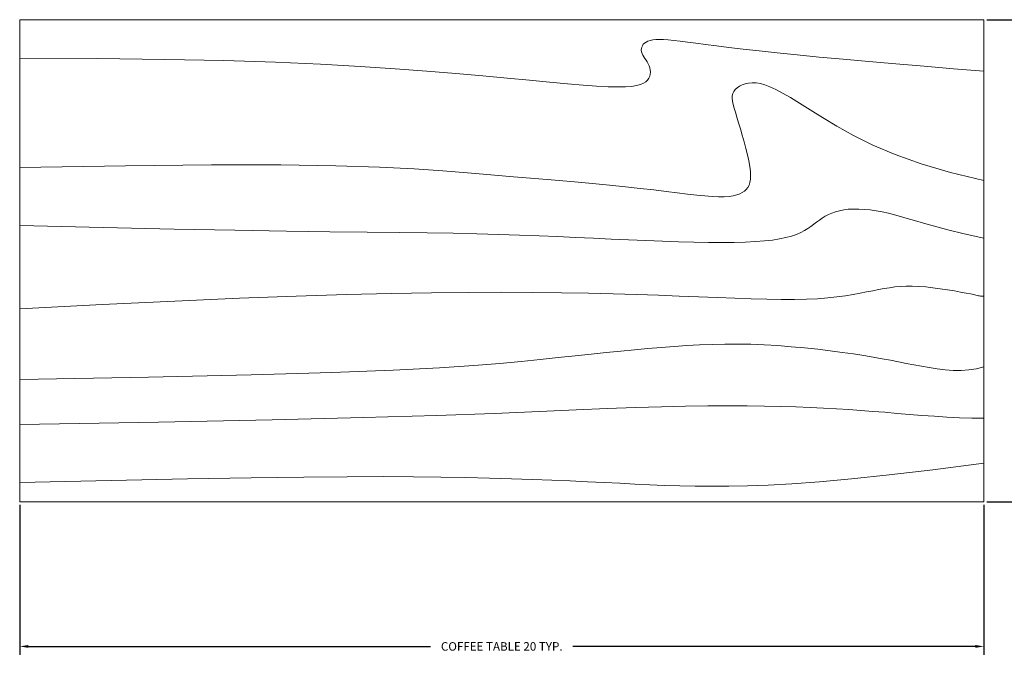
# Model space of a CAD drawing. Units: feet. Extents: x 2219 to 3039, y 1768 to 2369.
# Tile 8 of 16: x 2742.97 to 2763.81, y 2269.49 to 2283.32. Entities that reach past the tile are written whole.
import ezdxf

# ---------------------------------------------------------------- set-up
doc = ezdxf.new("R2010")
doc.units = ezdxf.units.FT
doc.layers.add('A-ANNO-DIMS', color=2, linetype='Continuous', lineweight=18)
doc.layers.add('A-FURN', color=8, linetype='Continuous', lineweight=18)
doc.styles.get("Standard").update_dxf_attribs({"font": 'arial.ttf'})
doc.dimstyles.get("Standard").update_dxf_attribs({"dimtxt": 0.18, "dimasz": 0.18, "dimexe": 0.18, "dimexo": 0.0625, "dimgap": 0.09, "dimtad": 0, "dimtih": 1, "dimtoh": 1, "dimdec": 4, "dimzin": 0, "dimdsep": 46, "dimtxsty": 'Standard', "dimcen": 0.09, "dimadec": 0, "dimazin": 0, "dimtfac": 1, "dimtdec": 4, "dimtofl": 0, "dimtmove": 0, "dimatfit": 3, "dimfxl": 1, "dimtolj": 1, "dimtzin": 0, "dimarcsym": 0})

# ---------------------------------------------------------------- blocks, each defined once
blk = doc.blocks.new('Table - Rectangular Woodgrain 60 x 30 in.')
for p, q in [((0, 0), (0, -30)), ((60, 0), (0, 0)), ((60, -30), (60, 0)), ((0, -30), (60, -30))]:
    blk.add_line(p, q)
for points in [[(0, -2.4), (4.8155, -2.418), (9.0302, -2.4688), (12.709, -2.5477), (15.9167, -2.65), (18.7181, -2.7711), (21.1781, -2.9063), (23.3616, -3.0508), (25.3333, -3.2), (27.1477, -3.3495), (28.8172, -3.4958), (30.3437, -3.636), (31.7291, -3.7667), (32.9756, -3.8849), (34.0849, -3.9875), (35.059, -4.0714), (35.9, -4.1334), (36.6114, -4.1711), (37.2041, -4.1854), (37.6906, -4.1779), (38.0833, -4.15), (38.3948, -4.1034), (38.6375, -4.0396), (38.8239, -3.9602), (38.9666, -3.8667), (39.0764, -3.7608), (39.1573, -3.6448), (39.2116, -3.521), (39.2416, -3.3917), (39.2498, -3.2593), (39.2385, -3.1261), (39.21, -2.9944), (39.1666, -2.8667), (39.111, -2.7447), (39.0468, -2.6281), (38.978, -2.5163), (38.9083, -2.4083), (38.8418, -2.3035), (38.7823, -2.201), (38.7337, -2.1001), (38.7, -2), (38.6844, -1.9003), (38.6875, -1.8021), (38.7094, -1.707), (38.75, -1.6167), (38.8094, -1.5326), (38.8875, -1.4563), (38.9844, -1.3893), (39.1, -1.3333), (39.2351, -1.2896), (39.3937, -1.2583), (39.5804, -1.2396), (39.8, -1.2333), (40.057, -1.2396), (40.3562, -1.2583), (40.7023, -1.2896), (41.1, -1.3333), (41.5547, -1.3895), (42.0755, -1.4573), (42.6721, -1.5361), (43.3542, -1.625), (44.1316, -1.7233), (45.014, -1.8302), (46.0114, -1.9449), (47.1333, -2.0667), (48.3862, -2.1947), (49.7625, -2.3281), (51.2513, -2.4663), (52.8416, -2.6083), (54.5226, -2.7535), (56.2833, -2.9011), (58.1127, -3.0501), (60, -3.2)], [(0, -9.2), (6.5759, -9.0858), (11.9385, -9.0365), (16.2527, -9.0418), (19.6833, -9.0917), (22.3952, -9.1759), (24.5531, -9.2844), (26.322, -9.4069), (27.8666, -9.5333), (29.3241, -9.6553), (30.7203, -9.7719), (32.0532, -9.8837), (33.3208, -9.9917), (34.5213, -10.0965), (35.6526, -10.199), (36.7128, -10.2999), (37.7, -10.4), (38.6129, -10.4996), (39.4531, -10.5969), (40.223, -10.6895), (40.925, -10.775), (41.5613, -10.8512), (42.1344, -10.9156), (42.6465, -10.966), (43.1, -11), (43.4976, -11.0158), (43.8437, -11.0136), (44.143, -10.9942), (44.4, -10.9583), (44.6195, -10.9069), (44.8062, -10.8406), (44.9648, -10.7603), (45.1, -10.6667), (45.2155, -10.5598), (45.3114, -10.4365), (45.3871, -10.2929), (45.4416, -10.125), (45.4743, -9.929), (45.4844, -9.7011), (45.4709, -9.4371), (45.4333, -9.1333), (45.3716, -8.7883), (45.2896, -8.4104), (45.1919, -8.0107), (45.0833, -7.6), (44.9685, -7.1893), (44.8521, -6.7896), (44.7388, -6.4117), (44.6333, -6.0667), (44.54, -5.7628), (44.4614, -5.4979), (44.4001, -5.2675), (44.3583, -5.0667), (44.3384, -4.8909), (44.3427, -4.7354), (44.3736, -4.5956), (44.4333, -4.4667), (44.5236, -4.3453), (44.6427, -4.2333), (44.7884, -4.1339), (44.9583, -4.05), (45.1501, -3.9849), (45.3614, -3.9417), (45.59, -3.9234), (45.8333, -3.9333), (46.0915, -3.9749), (46.3734, -4.0531), (46.6906, -4.1736), (47.0542, -4.3417), (47.4756, -4.5629), (47.9661, -4.8427), (48.5372, -5.1866), (49.2, -5.6), (49.9676, -6.0844), (50.8594, -6.625), (51.8965, -7.2031), (53.1, -7.8), (54.491, -8.3969), (56.0906, -8.975), (57.9199, -9.5156), (60, -10)], [(0, -12.8), (5.1847, -12.9322), (9.6213, -13.0323), (13.3963, -13.1059), (16.5958, -13.1583), (19.3063, -13.1952), (21.614, -13.2219), (23.6054, -13.2439), (25.3666, -13.2667), (26.9728, -13.2947), (28.4531, -13.3281), (29.8256, -13.3663), (31.1083, -13.4083), (32.3191, -13.4535), (33.476, -13.501), (34.597, -13.5501), (35.7, -13.6), (36.7984, -13.6497), (37.8875, -13.6979), (38.9578, -13.743), (40, -13.7833), (41.0047, -13.8174), (41.9625, -13.8438), (42.864, -13.8607), (43.7, -13.8667), (44.4631, -13.8604), (45.1552, -13.8417), (45.7801, -13.8104), (46.3416, -13.7667), (46.8439, -13.7104), (47.2906, -13.6417), (47.6858, -13.5604), (48.0333, -13.4667), (48.3375, -13.3608), (48.6042, -13.2448), (48.8396, -13.121), (49.05, -12.9917), (49.2417, -12.8593), (49.4208, -12.7261), (49.5937, -12.5944), (49.7667, -12.4667), (49.9452, -12.3451), (50.1323, -12.2313), (50.3303, -12.1268), (50.5416, -12.0333), (50.7686, -11.9524), (51.0135, -11.8854), (51.2788, -11.8341), (51.5666, -11.8), (51.8785, -11.7843), (52.2116, -11.7865), (52.562, -11.8059), (52.926, -11.8417), (53.2998, -11.8931), (53.6795, -11.9594), (54.0614, -12.0397), (54.4416, -12.1333), (54.8223, -12.2401), (55.2293, -12.3625), (55.6942, -12.5037), (56.2489, -12.6667), (56.9251, -12.8547), (57.7545, -13.0708), (58.7689, -13.3182), (60, -13.6)], [(0, -18), (5.124, -17.7273), (9.6609, -17.5057), (13.6705, -17.3303), (17.2125, -17.1958), (20.3467, -17.0973), (23.1328, -17.0297), (25.6307, -16.9878), (27.9, -16.9667), (29.9928, -16.9617), (31.9302, -16.9703), (33.7254, -16.9907), (35.3917, -17.0208), (36.9423, -17.0588), (38.3906, -17.1026), (39.7499, -17.1503), (41.0333, -17.2), (42.2519, -17.2496), (43.4073, -17.2969), (44.4986, -17.3395), (45.525, -17.375), (46.4858, -17.4012), (47.3802, -17.4156), (48.2074, -17.416), (48.9667, -17.4), (49.6583, -17.3662), (50.2872, -17.3167), (50.8595, -17.2547), (51.3812, -17.1833), (51.8584, -17.1057), (52.2971, -17.025), (52.7034, -16.9443), (53.0833, -16.8667), (53.443, -16.7951), (53.789, -16.7313), (54.128, -16.6768), (54.4666, -16.6334), (54.8115, -16.6024), (55.1693, -16.5854), (55.5465, -16.5841), (55.95, -16.6), (56.3828, -16.6337), (56.8346, -16.6823), (57.2915, -16.7418), (57.7396, -16.8084), (58.165, -16.878), (58.5539, -16.9469), (58.8924, -17.0111), (59.1666, -17.0667), (59.3679, -17.1107), (59.5078, -17.1438), (59.6032, -17.1675), (59.6708, -17.1833), (59.7275, -17.193), (59.7901, -17.1979), (59.8753, -17.1998), (60, -17.2)], [(0, -22.4), (8.0098, -22.2501), (14.4094, -22.1011), (19.4168, -21.9535), (23.25, -21.8083), (26.1269, -21.6663), (28.2656, -21.5281), (29.884, -21.3947), (31.2, -21.2667), (32.3967, -21.1448), (33.5172, -21.0292), (34.5697, -20.9198), (35.5625, -20.8167), (36.5037, -20.7198), (37.4015, -20.6292), (38.2642, -20.5448), (39.1, -20.4667), (39.9164, -20.3951), (40.7187, -20.3313), (41.5117, -20.2768), (42.3, -20.2333), (43.0883, -20.2024), (43.8812, -20.1854), (44.6836, -20.1841), (45.5, -20.2), (46.3328, -20.234), (47.1747, -20.2844), (48.0163, -20.3488), (48.8479, -20.425), (49.66, -20.5106), (50.4429, -20.6031), (51.1872, -20.7004), (51.8833, -20.8), (52.5246, -20.8999), (53.1166, -20.9995), (53.6681, -21.0983), (54.1875, -21.1958), (54.6834, -21.2919), (55.1646, -21.3859), (55.6394, -21.4777), (56.1167, -21.5667), (56.6028, -21.6515), (57.0961, -21.7266), (57.5929, -21.7852), (58.0896, -21.8208), (58.5823, -21.8268), (59.0674, -21.7964), (59.5412, -21.723), (60, -21.6)], [(0, -25.2), (8.6355, -25.0504), (15.7026, -24.9031), (21.4049, -24.7606), (25.9458, -24.625), (29.529, -24.4988), (32.3578, -24.3844), (34.6359, -24.284), (36.5667, -24.2), (38.3213, -24.1341), (39.9417, -24.0854), (41.437, -24.0523), (42.8167, -24.0333), (44.0901, -24.0268), (45.2667, -24.0313), (46.3557, -24.0451), (47.3667, -24.0667), (48.309, -24.0947), (49.1928, -24.1287), (50.0284, -24.168), (50.826, -24.2125), (51.5959, -24.2617), (52.3483, -24.3151), (53.0935, -24.3725), (53.8417, -24.4334), (54.6009, -24.497), (55.3699, -24.561), (56.1454, -24.6226), (56.9239, -24.6792), (57.7021, -24.7279), (58.4764, -24.7662), (59.2435, -24.7911), (60, -24.8)], [(0, -28.8), (5.6867, -28.6681), (10.45, -28.5698), (14.407, -28.5012), (17.675, -28.4584), (20.3711, -28.4374), (22.6125, -28.4344), (24.5164, -28.4455), (26.2, -28.4667), (27.762, -28.4947), (29.2276, -28.5281), (30.6033, -28.5663), (31.8958, -28.6084), (33.1118, -28.6535), (34.2578, -28.7011), (35.3405, -28.7501), (36.3666, -28.8), (37.3443, -28.8497), (38.288, -28.8974), (39.2137, -28.9412), (40.1375, -28.9792), (41.0753, -29.0093), (42.0432, -29.0297), (43.0572, -29.0384), (44.1333, -29.0333), (45.2936, -29.0114), (46.5843, -28.9641), (48.0579, -28.8816), (49.7666, -28.7542), (51.7629, -28.5721), (54.0989, -28.3255), (56.8272, -28.0048), (60, -27.6)]]:
    blk.add_lwpolyline(points)
blk = doc.blocks.new('*D28')
at = {"layer": 'A-ANNO-DIMS', "color": 0, "lineweight": -2, "transparency": 16777216}
for p, q in [((2742.974, 2273.061), (2742.974, 2269.883)), ((2763.375, 2273.061), (2763.375, 2269.883)), ((2743.154, 2270.063), (2751.669, 2270.063)), ((2763.195, 2270.063), (2754.679, 2270.063))]:
    blk.add_line(p, q, dxfattribs=at)
at = {"layer": 'A-ANNO-DIMS', "color": 0, "transparency": 16777216}
for points in [[(2743.154, 2270.093), (2743.154, 2270.033), (2742.974, 2270.063)], [(2763.195, 2270.093), (2763.195, 2270.033), (2763.375, 2270.063)]]:
    blk.add_solid(points, dxfattribs=at)
at = {"layer": 'Defpoints', "color": 0, "transparency": 16777216}
for p in [(2742.974, 2273.123), (2763.375, 2273.123), (2763.375, 2270.063)]:
    blk.add_point(p, dxfattribs=at)
at = {"layer": 'A-ANNO-DIMS', "color": 0, "transparency": 16777216, "insert": (2753.174, 2270.063), "char_height": 0.18, "attachment_point": 5}
blk.add_mtext('\\A1;COFFEE TABLE 20 TYP.', dxfattribs=at)
blk = doc.blocks.new('*D29')
at = {"layer": 'A-ANNO-DIMS', "color": 0, "lineweight": -2, "transparency": 16777216}
for p, q in [((2763.438, 2283.324), (2766.615, 2283.324)), ((2766.435, 2283.144), (2766.435, 2278.405)), ((2766.435, 2273.303), (2766.435, 2278.042)), ((2763.438, 2273.123), (2766.615, 2273.123))]:
    blk.add_line(p, q, dxfattribs=at)
at = {"layer": 'A-ANNO-DIMS', "color": 0, "transparency": 16777216}
for points in [[(2766.405, 2283.144), (2766.465, 2283.144), (2766.435, 2283.324)], [(2766.405, 2273.303), (2766.465, 2273.303), (2766.435, 2273.123)]]:
    blk.add_solid(points, dxfattribs=at)
at = {"layer": 'Defpoints', "color": 0, "transparency": 16777216}
for p in [(2763.375, 2283.324), (2766.435, 2283.324), (2763.375, 2273.123)]:
    blk.add_point(p, dxfattribs=at)
at = {"layer": 'A-ANNO-DIMS', "color": 0, "transparency": 16777216, "insert": (2766.435, 2278.224), "char_height": 0.18, "attachment_point": 5}
blk.add_mtext('\\A1;10 TYP.', dxfattribs=at)

msp = doc.modelspace()

# ---------------------------------------------------------------- block references
at = {"layer": 'A-FURN', "xscale": 0.3400232329989347, "yscale": 0.3400232329989347, "zscale": 0.3400232329989347}
msp.add_blockref('Table - Rectangular Woodgrain 60 x 30 in.', (2742.974, 2283.324), dxfattribs=at)

# ---------------------------------------------------------------- dimensions: what is measured, and where the dimension line sits
at = {"layer": 'A-ANNO-DIMS'}
dim = msp.add_linear_dim(base=(2766.435, 2283.324), p1=(2763.375, 2273.123), p2=(2763.375, 2283.324), angle=90, text='<> TYP.', dimstyle='Standard', override={"dimdec": 0, "dimlfac": 1, "dimrnd": 0, "dimzin": 0, "dimdsep": 46, "dimlunit": 2}, dxfattribs=at)
dim.commit()
dim.dimension.update_dxf_attribs({"geometry": '*D29', "text_midpoint": (2766.435, 2278.224)})
dim = msp.add_linear_dim(base=(2763.375, 2270.063), p1=(2742.974, 2273.123), p2=(2763.375, 2273.123), text='COFFEE TABLE <> TYP.', dimstyle='Standard', override={"dimdec": 0, "dimlfac": 1, "dimrnd": 0, "dimzin": 0, "dimdsep": 46, "dimlunit": 2}, dxfattribs=at)
dim.commit()
dim.dimension.update_dxf_attribs({"geometry": '*D28', "text_midpoint": (2753.174, 2270.063)})

doc.saveas('drawing.dxf')
